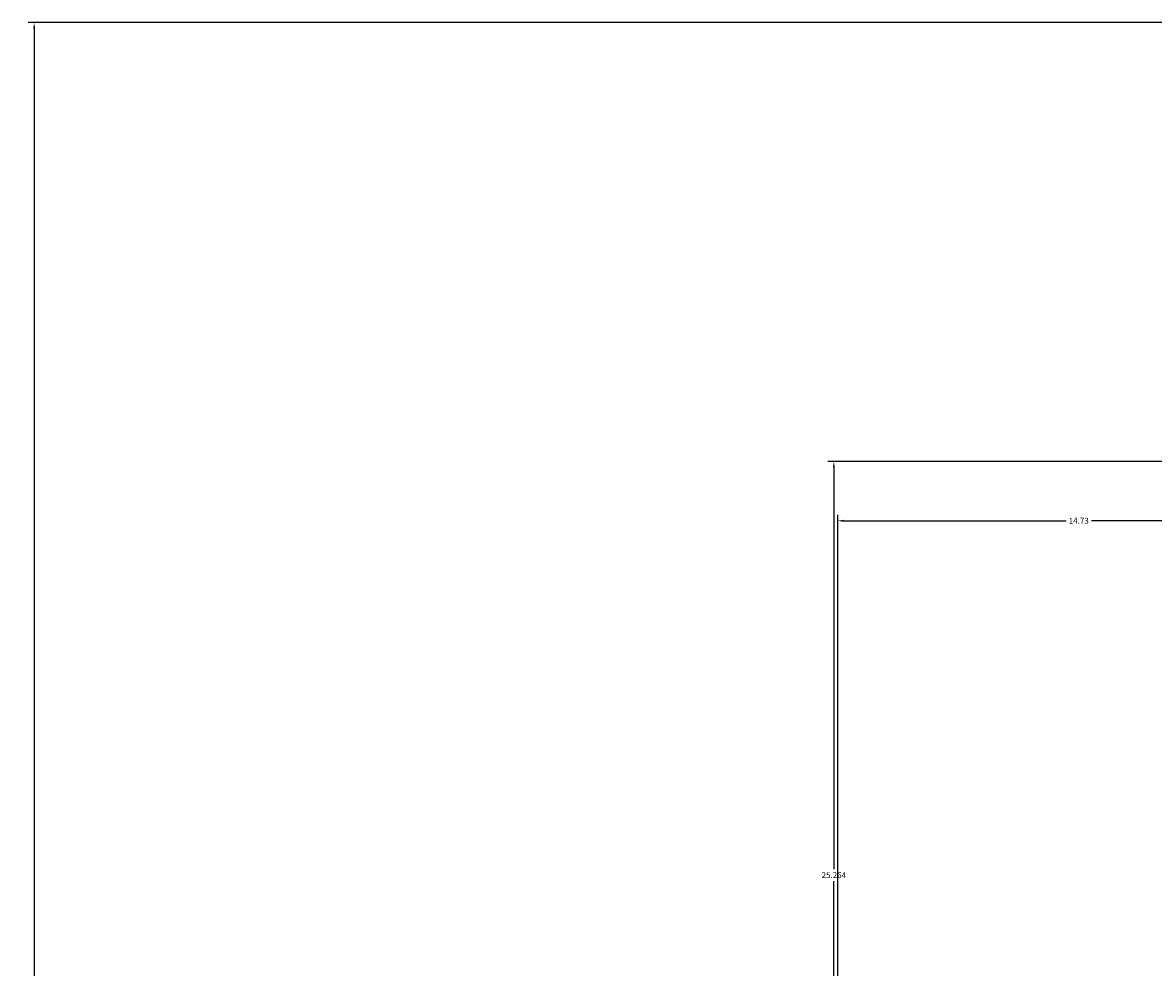
# Model space of a CAD drawing. Units: millimetres. Extents: x -11 to 280, y -4 to 208.
# Tile 14 of 55: x -10 to 24, y 164 to 193. Entities that reach past the tile are written whole.
import ezdxf

# ---------------------------------------------------------------- set-up
doc = ezdxf.new("R2010")
doc.units = ezdxf.units.MM
doc.layers.add('M-DIMS', color=2, linetype='Continuous', lineweight=18)
doc.styles.get("Standard").update_dxf_attribs({"font": 'arial.ttf'})
doc.dimstyles.get("Standard").update_dxf_attribs({"dimtxt": 0.18, "dimasz": 0.18, "dimexe": 0.18, "dimexo": 0.0625, "dimgap": 0.09, "dimtad": 0, "dimtih": 1, "dimtoh": 1, "dimdec": 4, "dimzin": 0, "dimdsep": 46, "dimtxsty": 'Standard', "dimcen": 0.09, "dimadec": 0, "dimazin": 0, "dimtfac": 1, "dimtdec": 4, "dimtofl": 0, "dimtmove": 0, "dimatfit": 3, "dimfxl": 1, "dimtolj": 1, "dimtzin": 0, "dimarcsym": 0})

# ---------------------------------------------------------------- blocks, each defined once
blk = doc.blocks.new('*D5')
at = {"layer": 'Defpoints', "color": 0, "transparency": 16777216}
for p in [(24.759, 192.645), (-10.087, 11.435), (261.686, 11.435)]:
    blk.add_point(p, dxfattribs=at)
at = {"layer": 'M-DIMS', "color": 0, "lineweight": -2, "transparency": 16777216}
for p, q in [((24.696, 192.645), (-10.267, 192.645)), ((-10.087, 192.465), (-10.087, 102.222)), ((-10.087, 11.615), (-10.087, 101.858)), ((261.624, 11.435), (-10.267, 11.435))]:
    blk.add_line(p, q, dxfattribs=at)
at = {"layer": 'M-DIMS', "color": 0, "transparency": 16777216}
for points in [[(-10.117, 192.465), (-10.057, 192.465), (-10.087, 192.645)], [(-10.117, 11.615), (-10.057, 11.615), (-10.087, 11.435)]]:
    blk.add_solid(points, dxfattribs=at)
at = {"layer": 'M-DIMS', "color": 0, "transparency": 16777216, "insert": (-10.087, 102.04), "char_height": 0.18, "attachment_point": 5}
blk.add_mtext('\\A1;181.2', dxfattribs=at)
blk = doc.blocks.new('*D8')
at = {"layer": 'Defpoints', "color": 0, "transparency": 16777216}
for p in [(29.201, 177.431), (14.47, 162.581), (29.201, 162.581)]:
    blk.add_point(p, dxfattribs=at)
at = {"layer": 'M-DIMS', "color": 0, "lineweight": -2, "transparency": 16777216}
for p, q in [((14.47, 162.644), (14.47, 177.611)), ((14.65, 177.431), (21.451, 177.431)), ((29.021, 177.431), (22.221, 177.431)), ((29.201, 162.644), (29.201, 177.611))]:
    blk.add_line(p, q, dxfattribs=at)
at = {"layer": 'M-DIMS', "color": 0, "transparency": 16777216}
for points in [[(14.65, 177.461), (14.65, 177.401), (14.47, 177.431)], [(29.021, 177.461), (29.021, 177.401), (29.201, 177.431)]]:
    blk.add_solid(points, dxfattribs=at)
at = {"layer": 'M-DIMS', "color": 0, "transparency": 16777216, "insert": (21.836, 177.431), "char_height": 0.18, "attachment_point": 5}
blk.add_mtext('\\A1;14.73', dxfattribs=at)
blk = doc.blocks.new('*D24')
at = {"layer": 'Defpoints', "color": 0, "transparency": 16777216}
for p in [(14.351, 179.241), (29.201, 179.241), (29.201, 153.977)]:
    blk.add_point(p, dxfattribs=at)
at = {"layer": 'M-DIMS', "color": 0, "lineweight": -2, "transparency": 16777216}
for p, q in [((29.139, 179.241), (14.171, 179.241)), ((14.351, 179.061), (14.351, 166.791)), ((14.351, 154.157), (14.351, 166.427)), ((29.139, 153.977), (14.171, 153.977))]:
    blk.add_line(p, q, dxfattribs=at)
at = {"layer": 'M-DIMS', "color": 0, "transparency": 16777216}
for points in [[(14.321, 179.061), (14.381, 179.061), (14.351, 179.241)], [(14.321, 154.157), (14.381, 154.157), (14.351, 153.977)]]:
    blk.add_solid(points, dxfattribs=at)
at = {"layer": 'M-DIMS', "color": 0, "transparency": 16777216, "insert": (14.351, 166.609), "char_height": 0.18, "attachment_point": 5}
blk.add_mtext('\\A1;25.264', dxfattribs=at)

msp = doc.modelspace()

# ---------------------------------------------------------------- dimensions: what is measured, and where the dimension line sits
at = {"layer": 'M-DIMS'}
for base, p1, p2, override, picture, middle in [((-10.0865, 11.4346), (24.7588, 192.645), (261.6863, 11.4346), {"dimdec": 1, "dimlfac": 1, "dimrnd": 0, "dimzin": 0, "dimdsep": 46, "dimlunit": 2}, '*D5', (-10.0865, 102.0398)), ((14.3515, 179.2412), (29.2015, 153.9768), (29.2015, 179.2412), {"dimdec": 3, "dimlfac": 1, "dimrnd": 0, "dimzin": 0, "dimdsep": 46, "dimlunit": 2}, '*D24', (14.3515, 166.609))]:
    dim = msp.add_linear_dim(base=base, p1=p1, p2=p2, angle=90, dimstyle='Standard', override=override, dxfattribs=at)
    dim.commit()
    dim.dimension.update_dxf_attribs({"geometry": picture, "text_midpoint": middle})
dim = msp.add_linear_dim(base=(29.2015, 177.4314), p1=(14.4701, 162.5814), p2=(29.2015, 162.5814), dimstyle='Standard', override={"dimdec": 2, "dimlfac": 1, "dimrnd": 0, "dimzin": 0, "dimdsep": 46, "dimlunit": 2}, dxfattribs=at)
dim.commit()
dim.dimension.update_dxf_attribs({"geometry": '*D8', "text_midpoint": (21.8358, 177.4314)})

doc.saveas('drawing.dxf')
